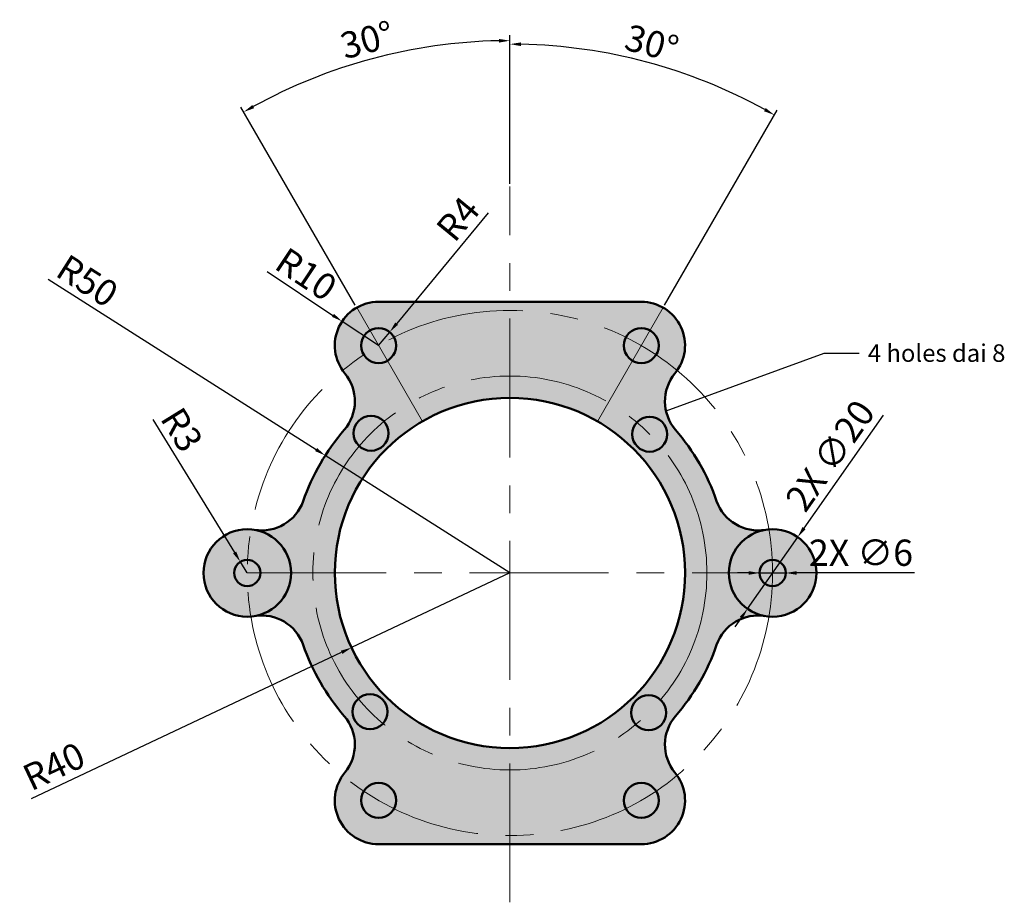
# Model space of a CAD drawing. Units: millimetres. Extents: x 3166 to 3391, y 1547 to 1748.
import ezdxf
from ezdxf import colors
from ezdxf.entities.mleader import LeaderData, LeaderLine
from ezdxf.math import Vec2, Vec3

# ---------------------------------------------------------------- set-up
doc = ezdxf.new("R2010")
doc.units = ezdxf.units.MM
doc.linetypes.add('CENTER', pattern=[50.8, 31.75, -6.35, 6.35, -6.35])
for name, color, linetype, lineweight in [('M-CNTR', 240, 'CENTER', 18), ('M-DIMS', 2, 'Continuous', 25), ('M-HATC', 8, 'Continuous', 18), ('M-OUTL', 7, 'Continuous', 50), ('M-TEXT', 7, 'Continuous', 25)]:
    doc.layers.add(name, color=color, linetype=linetype, lineweight=lineweight)
doc.styles.get("Standard").update_dxf_attribs({"font": 'arial.ttf'})
doc.dimstyles.new('ISO-25', dxfattribs={"dimtxt": 6, "dimasz": 2.5, "dimexe": 1.25, "dimexo": 0.625, "dimtad": 1, "dimtxsty": 'Standard', "dimcen": 2.5, "dimadec": 0, "dimazin": 0, "dimtfac": 1, "dimtmove": 0, "dimatfit": 3, "dimfxl": 1, "dimarcsym": 0})

# ---------------------------------------------------------------- blocks, each defined once
blk = doc.blocks.new('*D1')
at = {"layer": 'Defpoints', "color": 0, "transparency": 16777216}
for p in [(3277.67, 1622.08), (3241.49, 1605.02)]:
    blk.add_point(p, dxfattribs=at)
at = {"layer": 'M-DIMS', "color": 0, "lineweight": -2, "transparency": 16777216}
for p, q in [((3277.67, 1622.08), (3241.49, 1605.02)), ((3168.36, 1570.54), (3239.23, 1603.95))]:
    blk.add_line(p, q, dxfattribs=at)
at = {"layer": 'M-DIMS', "color": 0, "transparency": 16777216}
blk.add_solid([(3239.05, 1604.33), (3239.4, 1603.58), (3241.49, 1605.02)], dxfattribs=at)
at = {"layer": 'M-DIMS', "color": 0, "transparency": 16777216, "insert": (3173.82, 1577.2), "char_height": 6, "attachment_point": 5, "rotation": 25.2427}
blk.add_mtext('R40', dxfattribs=at)
blk = doc.blocks.new('*D2')
at = {"layer": 'Defpoints', "color": 0, "transparency": 16777216}
for p in [(3235.49, 1648.93), (3277.67, 1622.08)]:
    blk.add_point(p, dxfattribs=at)
at = {"layer": 'M-DIMS', "color": 0, "lineweight": -2, "transparency": 16777216}
for p, q in [((3172.19, 1689.24), (3233.38, 1650.28)), ((3277.67, 1622.08), (3235.49, 1648.93))]:
    blk.add_line(p, q, dxfattribs=at)
at = {"layer": 'M-DIMS', "color": 0, "transparency": 16777216}
blk.add_solid([(3233.61, 1650.63), (3233.16, 1649.92), (3235.49, 1648.93)], dxfattribs=at)
at = {"layer": 'M-DIMS', "color": 0, "transparency": 16777216, "insert": (3180.74, 1688.17), "char_height": 6, "attachment_point": 5, "rotation": 327.514}
blk.add_mtext('R50', dxfattribs=at)
blk = doc.blocks.new('*D3')
at = {"layer": 'Defpoints', "color": 0, "transparency": 16777216}
for p in [(3239.33, 1679.56), (3247.67, 1674.04)]:
    blk.add_point(p, dxfattribs=at)
at = {"layer": 'M-DIMS', "color": 0, "lineweight": -2, "transparency": 16777216}
for p, q in [((3222.18, 1690.92), (3237.25, 1680.94)), ((3247.67, 1674.04), (3239.33, 1679.56))]:
    blk.add_line(p, q, dxfattribs=at)
at = {"layer": 'M-DIMS', "color": 0, "transparency": 16777216}
blk.add_solid([(3237.48, 1681.29), (3237.02, 1680.6), (3239.33, 1679.56)], dxfattribs=at)
at = {"layer": 'M-DIMS', "color": 0, "transparency": 16777216, "insert": (3230.71, 1689.7), "char_height": 6, "attachment_point": 5, "rotation": 326.4806}
blk.add_mtext('R10', dxfattribs=at)
blk = doc.blocks.new('*D4')
at = {"layer": 'Defpoints', "color": 0, "transparency": 16777216}
for p in [(3250.21, 1677.13), (3247.67, 1674.04)]:
    blk.add_point(p, dxfattribs=at)
at = {"layer": 'M-DIMS', "color": 0, "lineweight": -2, "transparency": 16777216}
for p, q in [((3272.67, 1704.38), (3251.8, 1679.06)), ((3247.67, 1674.04), (3250.21, 1677.13))]:
    blk.add_line(p, q, dxfattribs=at)
at = {"layer": 'M-DIMS', "color": 0, "transparency": 16777216}
blk.add_solid([(3251.48, 1679.32), (3252.12, 1678.79), (3250.21, 1677.13)], dxfattribs=at)
at = {"layer": 'M-DIMS', "color": 0, "transparency": 16777216, "insert": (3266.4, 1702.48), "char_height": 6, "attachment_point": 5, "rotation": 50.5119}
blk.add_mtext('R4', dxfattribs=at)
blk = doc.blocks.new('*D5')
at = {"layer": 'Defpoints', "color": 0, "transparency": 16777216}
for p in [(3216.09, 1624.63), (3217.67, 1622.08)]:
    blk.add_point(p, dxfattribs=at)
at = {"layer": 'M-DIMS', "color": 0, "lineweight": -2, "transparency": 16777216}
for p, q in [((3196.07, 1657.12), (3214.78, 1626.76)), ((3217.67, 1622.08), (3216.09, 1624.63))]:
    blk.add_line(p, q, dxfattribs=at)
at = {"layer": 'M-DIMS', "color": 0, "transparency": 16777216}
blk.add_solid([(3215.14, 1626.98), (3214.43, 1626.54), (3216.09, 1624.63)], dxfattribs=at)
at = {"layer": 'M-DIMS', "color": 0, "transparency": 16777216, "insert": (3202.07, 1654.41), "char_height": 6, "attachment_point": 5, "rotation": 301.6517}
blk.add_mtext('R3', dxfattribs=at)
blk = doc.blocks.new('*D6')
at = {"layer": 'Defpoints', "color": 0, "transparency": 16777216}
for p in [(3256.55, 1741.85), (3277.67, 1710.4), (3242.67, 1682.7), (3257.67, 1656.72), (3277.67, 1546.83)]:
    blk.add_point(p, dxfattribs=at)
at = {"layer": 'M-DIMS', "color": 0, "lineweight": -2, "transparency": 16777216}
for p, q in [((3277.67, 1711.02), (3277.67, 1744.94)), ((3242.35, 1683.24), (3216.23, 1728.48))]:
    blk.add_line(p, q, dxfattribs=at)
blk.add_arc((3277.67, 1622.08), 121.62, 91.1778, 118.8222, dxfattribs=at)
at = {"layer": 'M-DIMS', "color": 0, "transparency": 16777216}
for points in [[(3275.16, 1744.09), (3275.17, 1743.25), (3277.67, 1743.69)], [(3219.24, 1728.27), (3218.83, 1728.99), (3216.86, 1727.4)]]:
    blk.add_solid(points, dxfattribs=at)
at = {"layer": 'M-DIMS', "color": 0, "transparency": 16777216, "insert": (3245.24, 1743.12), "char_height": 6, "attachment_point": 5, "rotation": 15}
blk.add_mtext('30°', dxfattribs=at)
blk = doc.blocks.new('*D7')
at = {"layer": 'Defpoints', "color": 0, "transparency": 16777216}
for p in [(3318.99, 1735.61), (3277.67, 1710.4), (3312.67, 1682.7), (3297.67, 1656.72), (3277.67, 1546.83)]:
    blk.add_point(p, dxfattribs=at)
at = {"layer": 'M-DIMS', "color": 0, "lineweight": -2, "transparency": 16777216}
for p, q in [((3277.67, 1711.02), (3277.67, 1744.15)), ((3312.98, 1683.24), (3338.7, 1727.8))]:
    blk.add_line(p, q, dxfattribs=at)
blk.add_arc((3277.67, 1622.08), 120.82, 61.1856, 88.8144, dxfattribs=at)
at = {"layer": 'M-DIMS', "color": 0, "transparency": 16777216}
for points in [[(3280.16, 1742.46), (3280.17, 1743.29), (3277.67, 1742.9)], [(3336.1, 1728.3), (3335.7, 1727.58), (3338.08, 1726.71)]]:
    blk.add_solid(points, dxfattribs=at)
at = {"layer": 'M-DIMS', "color": 0, "transparency": 16777216, "insert": (3309.89, 1742.35), "char_height": 6, "attachment_point": 5, "rotation": 345}
blk.add_mtext('30°', dxfattribs=at)
blk = doc.blocks.new('FLANGE-HOLE-D8')
blk.add_circle((0, 0), 4)
blk = doc.blocks.new('FLANGE-SIDE-LUG-D20-D6')
for radius in [10, 3]:
    blk.add_circle((0, 0), radius)
blk = doc.blocks.new('*D10')
at = {"layer": 'Defpoints', "color": 0, "transparency": 16777216}
for p in [(3334.67, 1622.08), (3340.67, 1622.08)]:
    blk.add_point(p, dxfattribs=at)
at = {"layer": 'M-DIMS', "color": 0, "lineweight": -2, "transparency": 16777216}
for p, q in [((3332.17, 1622.08), (3329.67, 1622.08)), ((3334.67, 1622.08), (3340.67, 1622.08)), ((3370.05, 1622.08), (3343.17, 1622.08))]:
    blk.add_line(p, q, dxfattribs=at)
at = {"layer": 'M-DIMS', "color": 0, "transparency": 16777216}
for points in [[(3332.17, 1622.5), (3332.17, 1621.66), (3334.67, 1622.08)], [(3343.17, 1622.49), (3343.17, 1621.66), (3340.67, 1622.08)]]:
    blk.add_solid(points, dxfattribs=at)
at = {"layer": 'M-DIMS', "color": 0, "transparency": 16777216, "insert": (3357.86, 1625.93), "char_height": 6, "attachment_point": 5, "rotation": 359.9948}
blk.add_mtext('2X ∅6', dxfattribs=at)
blk = doc.blocks.new('*D11')
at = {"layer": 'Defpoints', "color": 0, "transparency": 16777216}
for p in [(3343.4, 1630.27), (3331.93, 1613.89)]:
    blk.add_point(p, dxfattribs=at)
at = {"layer": 'M-DIMS', "color": 0, "lineweight": -2, "transparency": 16777216}
for p, q in [((3362.92, 1658.14), (3344.84, 1632.32)), ((3331.93, 1613.89), (3343.4, 1630.27)), ((3330.5, 1611.84), (3329.06, 1609.79))]:
    blk.add_line(p, q, dxfattribs=at)
at = {"layer": 'M-DIMS', "color": 0, "transparency": 16777216}
for points in [[(3344.5, 1632.56), (3345.18, 1632.08), (3343.4, 1630.27)], [(3330.16, 1612.08), (3330.84, 1611.6), (3331.93, 1613.89)]]:
    blk.add_solid(points, dxfattribs=at)
at = {"layer": 'M-DIMS', "color": 0, "transparency": 16777216, "insert": (3351.44, 1648.47), "char_height": 6, "attachment_point": 5, "rotation": 54.9989}
blk.add_mtext('2X ∅20', dxfattribs=at)

msp = doc.modelspace()

# ---------------------------------------------------------------- hatches: boundary and pattern name
at = {"layer": 'M-HATC'}
h = msp.add_hatch(color=256, dxfattribs=at)
h.set_gradient(color1=(0, 255, 255), color2=(255, 255, 0), tint=1)
h.paths.add_polyline_path([(3247.667, 1684.04, 0.634583), (3239.961, 1667.666, -0.3659774), (3239.824, 1654.757, 0.0946323), (3230.445, 1638.512, -0.3659774), (3219.334, 1631.938, -0.3659774), (3227.667, 1622.078, -0.3659774), (3219.334, 1612.218, -0.3659774), (3230.445, 1605.645, 0.0946323), (3239.824, 1589.399, -0.3659774), (3239.961, 1576.49, 0.634583), (3247.667, 1560.117), (3307.667, 1560.117, 0.634583), (3315.373, 1576.49, -0.3659774), (3315.51, 1589.399, 0.0946323), (3324.889, 1605.645, -0.3659774), (3336, 1612.218, -0.3659774), (3327.667, 1622.078, -0.3659774), (3336, 1631.938, -0.3659774), (3324.889, 1638.512, 0.0946323), (3315.51, 1654.757, -0.3659774), (3315.373, 1667.666, 0.634583), (3307.667, 1684.04)])
h.paths.add_polyline_path([(3243.667, 1674.04, -1), (3251.667, 1674.04, -1)], flags=16)
h.paths.add_polyline_path([(3317.667, 1622.078, -1), (3237.667, 1622.078, -1)], flags=16)
h.paths.add_polyline_path([(3249.961, 1654.012, -1), (3241.961, 1654.012, -1)], flags=16)
h.paths.add_polyline_path([(3303.667, 1674.04, -1), (3311.667, 1674.04, -1)], flags=16)
h.paths.add_polyline_path([(3313.601, 1653.784, -1), (3305.601, 1653.784, -1)], flags=16)
h.paths.add_polyline_path([(3249.733, 1590.373, -1), (3241.733, 1590.373, -1)], flags=16)
h.paths.add_polyline_path([(3313.372, 1590.145, -1), (3305.372, 1590.145, -1)], flags=16)
h.paths.add_polyline_path([(3251.667, 1570.117, -1), (3243.667, 1570.117, -1)], flags=16)
h.paths.add_polyline_path([(3311.667, 1570.117, -1), (3303.667, 1570.117, -1)], flags=16)
h = msp.add_hatch(color=256, dxfattribs=at)
h.set_gradient(color1=(147, 39, 143), color2=(199, 200, 202), tint=1, name='SPHERICAL')
h.paths.add_polyline_path([(3243.667, 1674.04, 1), (3251.667, 1674.04, 1)])
h = msp.add_hatch(color=256, dxfattribs=at)
h.set_gradient(color1=(147, 39, 143), color2=(199, 200, 202), tint=1, name='SPHERICAL')
h.paths.add_polyline_path([(3311.667, 1674.04, 1), (3303.667, 1674.04, 1)])
h = msp.add_hatch(color=256, dxfattribs=at)
h.set_gradient(color1=(147, 39, 143), color2=(199, 200, 202), tint=1, name='SPHERICAL')
h.paths.add_polyline_path([(3241.961, 1654.012, 1), (3249.961, 1654.012, 1)])
h = msp.add_hatch(color=256, dxfattribs=at)
h.set_gradient(color1=(147, 39, 143), color2=(199, 200, 202), tint=1, name='SPHERICAL')
h.paths.add_polyline_path([(3313.601, 1653.784, 1), (3305.601, 1653.784, 1)])
h = msp.add_hatch(color=256, dxfattribs=at)
h.set_gradient(color1=(255, 255, 255), color2=(248, 153, 30), tint=1, name='INVSPHERICAL')
h.paths.add_polyline_path([(3207.667, 1622.078, 1), (3227.667, 1622.078, 1)])
h.paths.add_polyline_path([(3220.667, 1622.078, -1), (3214.667, 1622.078, -1)], flags=16)
h.paths.add_polyline_path([(3327.667, 1622.078, 1), (3347.667, 1622.078, 1)])
h.paths.add_polyline_path([(3340.667, 1622.078, -1), (3334.667, 1622.078, -1)], flags=16)
h = msp.add_hatch(color=256, dxfattribs=at)
h.set_gradient(color1=(147, 39, 143), color2=(199, 200, 202), tint=1, name='SPHERICAL')
h.paths.add_polyline_path([(3214.667, 1622.078, 1), (3220.667, 1622.078, 1)])
h = msp.add_hatch(color=256, dxfattribs=at)
h.set_gradient(color1=(147, 39, 143), color2=(199, 200, 202), tint=1, name='SPHERICAL')
h.paths.add_polyline_path([(3340.667, 1622.078, 1), (3334.667, 1622.078, 1)])
h = msp.add_hatch(color=256, dxfattribs=at)
h.set_gradient(color1=(147, 39, 143), color2=(199, 200, 202), tint=1, name='SPHERICAL')
h.paths.add_polyline_path([(3249.733, 1590.373, 1), (3241.733, 1590.373, 1)])
h = msp.add_hatch(color=256, dxfattribs=at)
h.set_gradient(color1=(147, 39, 143), color2=(199, 200, 202), tint=1, name='SPHERICAL')
h.paths.add_polyline_path([(3305.372, 1590.145, 1), (3313.372, 1590.145, 1)])
h = msp.add_hatch(color=256, dxfattribs=at)
h.set_gradient(color1=(147, 39, 143), color2=(199, 200, 202), tint=1, name='SPHERICAL')
h.paths.add_polyline_path([(3251.667, 1570.117, 1), (3243.667, 1570.117, 1)])
h = msp.add_hatch(color=256, dxfattribs=at)
h.set_gradient(color1=(147, 39, 143), color2=(199, 200, 202), tint=1, name='SPHERICAL')
h.paths.add_polyline_path([(3311.667, 1570.117, 1), (3303.667, 1570.117, 1)])

# ---------------------------------------------------------------- linework, layer by layer
at = {"layer": 'M-CNTR'}
for p, q in [((3277.667, 1546.834), (3277.667, 1710.398)), ((3257.667, 1656.719), (3242.667, 1682.7)), ((3297.667, 1656.719), (3312.667, 1682.7)), ((3217.667, 1622.078), (3337.667, 1622.078))]:
    msp.add_line(p, q, dxfattribs=at)
for radius in [60, 45]:
    msp.add_circle((3277.667, 1622.078), radius, dxfattribs=at)
at = {"layer": 'M-OUTL'}
for p, q in [((3247.667, 1684.04), (3307.667, 1684.04)), ((3247.667, 1560.117), (3307.667, 1560.117))]:
    msp.add_line(p, q, dxfattribs=at)
msp.add_circle((3277.667, 1622.078), 40, dxfattribs=at)
for centre, radius, start, end in [((3247.667, 1674.04), 10, 90, 219.59407), ((3307.667, 1674.04), 10, 320.40593, 90), ((3232.255, 1661.293), 10, 319.18814, 39.59407), ((3323.078, 1661.293), 10, 140.40593, 220.81186), ((3277.667, 1622.078), 50, 139.18814, 160.81186), ((3277.667, 1622.078), 50, 19.18814, 40.81186), ((3221, 1641.799), 10, 260.40593, 340.81186), ((3334.334, 1641.799), 10, 199.18814, 279.59407), ((3221, 1602.358), 10, 19.18814, 99.59407), ((3334.334, 1602.358), 10, 80.40593, 160.81186), ((3277.667, 1622.078), 50, 199.18814, 220.81186), ((3277.667, 1622.078), 50, 319.18814, 340.81186), ((3232.255, 1582.864), 10, 320.40593, 40.81186), ((3323.078, 1582.864), 10, 139.18814, 219.59407), ((3247.667, 1570.117), 10, 140.40593, 270), ((3307.667, 1570.117), 10, 270, 39.59407)]:
    msp.add_arc(centre, radius, start, end, dxfattribs=at)

# ---------------------------------------------------------------- block references
for name, p in [('FLANGE-HOLE-D8', (3247.667, 1674.04)), ('FLANGE-HOLE-D8', (3307.667, 1674.04)), ('FLANGE-HOLE-D8', (3245.961, 1654.012)), ('FLANGE-HOLE-D8', (3309.601, 1653.784)), ('FLANGE-SIDE-LUG-D20-D6', (3217.667, 1622.078)), ('FLANGE-SIDE-LUG-D20-D6', (3337.667, 1622.078)), ('FLANGE-HOLE-D8', (3245.733, 1590.373)), ('FLANGE-HOLE-D8', (3309.372, 1590.145)), ('FLANGE-HOLE-D8', (3247.667, 1570.117)), ('FLANGE-HOLE-D8', (3307.667, 1570.117))]:
    msp.add_blockref(name, p, dxfattribs=at)

# ---------------------------------------------------------------- dimensions: what is measured, and where the dimension line sits
at = {"layer": 'M-DIMS'}
for base, line1, line2, picture, middle in [((3256.548, 1741.847), ((3277.667, 1546.834), (3277.667, 1710.398)), ((3257.667, 1656.719), (3242.667, 1682.7)), '*D6', (3245.235, 1743.115)), ((3318.99, 1735.614), ((3297.667, 1656.719), (3312.667, 1682.7)), ((3277.667, 1546.834), (3277.667, 1710.398)), '*D7', (3309.893, 1742.348))]:
    dim = msp.add_angular_dim_2l(base=base, line1=line1, line2=line2, dimstyle='ISO-25', override={"dimclrd": 0, "dimclre": 0, "dimclrt": 0}, dxfattribs=at)
    dim.commit()
    dim.dimension.update_dxf_attribs({"geometry": picture, "text_midpoint": middle})
for center, mpoint, picture, middle in [((3247.667, 1674.04), (3250.211, 1677.127), '*D4', (3269.199, 1700.172)), ((3277.667, 1622.078), (3235.491, 1648.933), '*D2', (3178.76, 1685.055)), ((3217.667, 1622.078), (3216.093, 1624.632), '*D5', (3198.932, 1652.469)), ((3277.667, 1622.078), (3241.486, 1605.02), '*D1', (3175.398, 1573.861))]:
    dim = msp.add_radius_dim(center=center, mpoint=mpoint, dimstyle='ISO-25', override={"dimclrd": 0, "dimclre": 0, "dimclrt": 0}, dxfattribs=at)
    dim.commit()
    dim.dimension.update_dxf_attribs({"geometry": picture, "text_midpoint": middle, "dimtype": 164})
dim = msp.add_radius_dim(center=(3247.667, 1674.04), mpoint=(3239.33, 1679.562), dimstyle='ISO-25', override={"dimclrd": 0, "dimclre": 0, "dimclrt": 0}, dxfattribs=at)
dim.commit()
dim.dimension.update_dxf_attribs({"geometry": '*D3', "text_midpoint": (3230.709, 1689.696)})
dim = msp.add_diameter_dim_2p(p1=(3331.931, 1613.887), p2=(3343.403, 1630.27), text='2X <>', dimstyle='ISO-25', override={"dimdec": 0, "dimlfac": 1, "dimrnd": 0, "dimzin": 0, "dimdsep": 46, "dimlunit": 2}, dxfattribs=at)
dim.commit()
dim.dimension.update_dxf_attribs({"geometry": '*D11', "text_midpoint": (3354.596, 1646.254)})
dim = msp.add_diameter_dim_2p(p1=(3334.667, 1622.079), p2=(3340.667, 1622.078), text='2X <>', dimstyle='ISO-25', override={"dimdec": 0, "dimlfac": 1, "dimrnd": 0, "dimzin": 0, "dimdsep": 46, "dimlunit": 2}, dxfattribs=at)
dim.commit()
dim.dimension.update_dxf_attribs({"geometry": '*D10', "text_midpoint": (3357.858, 1622.076), "dimtype": 163})

# ---------------------------------------------------------------- leaders
at = {"layer": 'M-TEXT'}
ml = msp.add_multileader_mtext('Standard', dxfattribs=at)
ml.set_content('4 holes dai 8', color=256)
ml.set_leader_properties()
ml.build(insert=Vec2(0, 0))
ctx = ml.context
ctx.base_point, ctx.plane_origin = Vec3(3357.424, 1672.278), Vec3(3309.601, 1657.784)
notes = []
notes.append((ctx, [(0, (1, 1, 0), (3349.424, 1672.278), (1, 0), 8, [(0, [(3309.601, 1657.784)], 0, [])])]))
ctx.mtext.insert, ctx.mtext.flow_direction = Vec3(3359.424, 1674.312), 5
for ctx, leaders in notes:
    for number, flags, end, landing, length, lines in leaders:
        leader = LeaderData()
        leader.index, (leader.has_last_leader_line, leader.has_dogleg_vector, leader.attachment_direction) = number, flags
        leader.last_leader_point, leader.dogleg_vector, leader.dogleg_length = Vec3(end), Vec3(landing), length
        for number, points, colour, breaks in lines:
            line = LeaderLine()
            line.index, line.vertices, line.color, line.breaks = number, Vec3.list(points), colors.encode_raw_color(colour), breaks
            leader.lines.append(line)
        ctx.leaders.append(leader)

doc.saveas('drawing.dxf')
